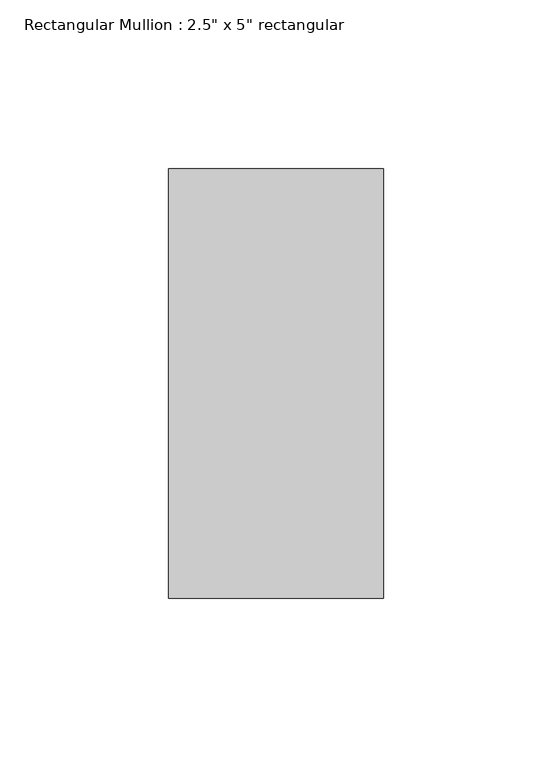
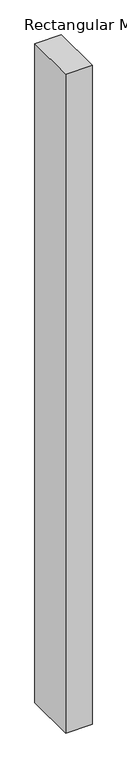
"""IFC4 building model written with IfcOpenShell, lengths in millimetres: member geometry."""

from ifc_helpers import new_model, si_unit, frame, origin, place, context, project, spatial, polyline, outline, extrude, source, transform, mapped, element, save


def member_b06f4f27(model_context):
    return source(origin(), model_context, "Body", "SweptSolid", [
        extrude(outline(polyline([(31.75, 63.5), (31.75, -63.5), (-31.75, -63.5), (-31.75, 63.5), (31.75, 63.5)])), frame((0.0, 0.0, -1668.686135), z_axis=(0.0, 0.0, 1.0), x_axis=(1.0, 0.0, 0.0)), (0.0, 0.0, 1.0), 1668.686135),
    ])


if __name__ == "__main__":
    model = new_model("IFC4")
    model_context = context("Model", 3, world=origin())
    ifc_project = project(units=[si_unit("LENGTHUNIT", "METRE", prefix="MILLI")], contexts=[model_context])
    site = spatial("IfcSite", under=ifc_project)
    building = spatial("IfcBuilding", under=site)
    placement = place(None, origin())
    member_shape = member_b06f4f27(model_context)
    element("IfcMember", 1, ObjectType="Rectangular Mullion : 2.5\" x 5\" rectangular", at=placement, inside=building, context=model_context, shape_type="MappedRepresentation", body=[
        mapped(member_shape, transform((0.0, 0.0, 0.0), x_axis=(1.0, 0.0, 0.0), y_axis=(0.0, 1.0, 0.0), z_axis=(0.0, 0.0, 1.0))),
    ])
    save(model, "model.ifc")

# Revit data of these elements
# Type "Rectangular Mullion : 2.5\" x 5\" rectangular"
#   built-in parameter 1007304 = 0.416667 (stored number, unit not read)
#   built-in parameter 1007301 = 0.104167 (stored number, unit not read)
#   built-in parameter 1007300 = 0.104167 (stored number, unit not read)
# Element 1 (IfcMember, "Rectangular Mullion : 2.5\" x 5\" rectangular")
#   Materials on its faces: "Aluminum"
# Materials
#   "Aluminum": class "Metal", colour RGB 247 247 247, transparency 0, Description = "Aluminum 6061", Cost = 0
